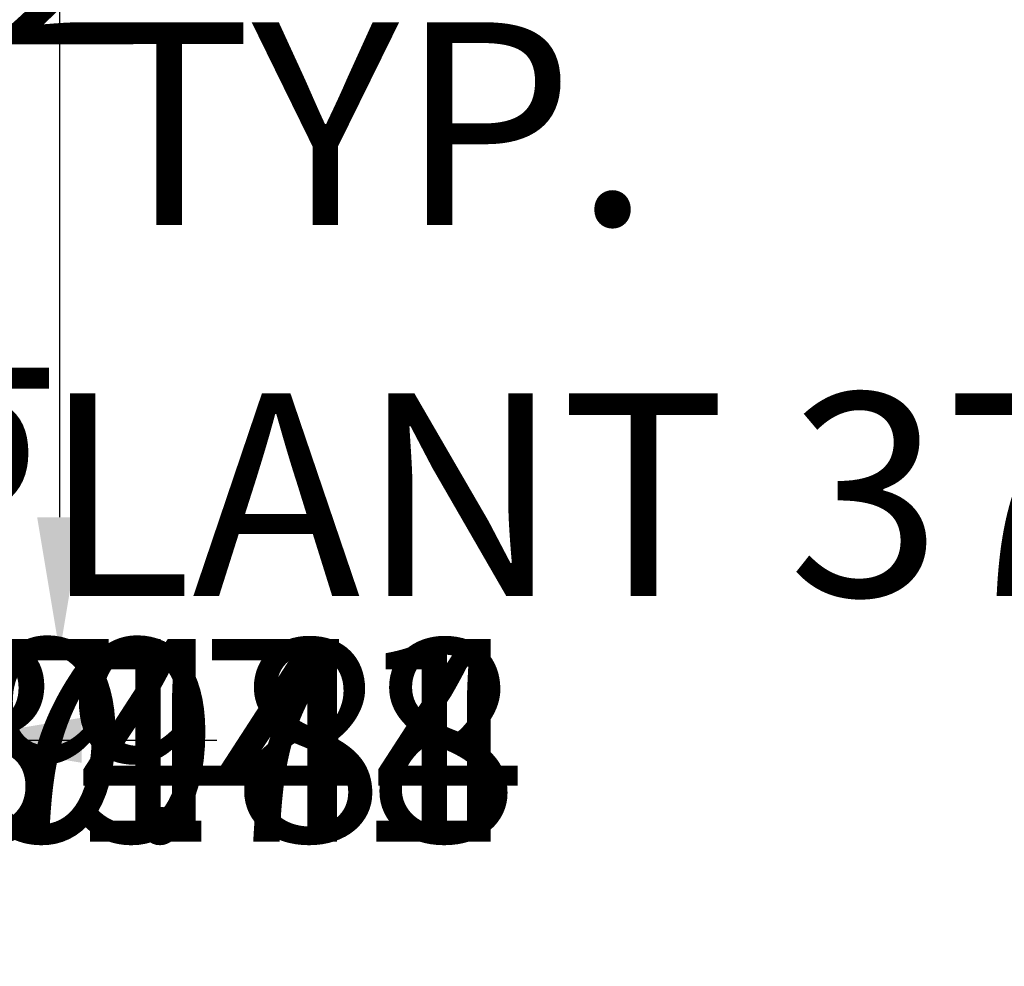
# Model space of a CAD drawing. Units: inches. Extents: x -307 to 2141, y -58 to 895.
# Tile 26 of 28: x 933 to 1283, y -44 to 292. Entities that reach past the tile are written whole.
import ezdxf

# ---------------------------------------------------------------- set-up
doc = ezdxf.new("R2010")
doc.units = ezdxf.units.IN
doc.header["$MEASUREMENT"] = 0
doc.layers.add('A-ANNO-DIMS', color=2, linetype='Continuous', lineweight=18)
doc.styles.get("Standard").update_dxf_attribs({"font": 'arial.ttf'})
doc.dimstyles.get("Standard").update_dxf_attribs({"dimtxt": 72, "dimasz": 48, "dimexe": 0.18, "dimexo": 0.0625, "dimgap": 0.09, "dimtad": 0, "dimtih": 1, "dimtoh": 1, "dimdec": 0, "dimrnd": 48, "dimzin": 0, "dimdsep": 46, "dimlunit": 3, "dimtxsty": 'Standard', "dimcen": 0.09, "dimadec": 0, "dimazin": 0, "dimtfac": 1, "dimtdec": 0, "dimtofl": 0, "dimtmove": 0, "dimatfit": 3, "dimfxl": 1, "dimtolj": 1, "dimtzin": 0, "dimarcsym": 0})

# ---------------------------------------------------------------- blocks, each defined once
blk = doc.blocks.new('*D34')
at = {"layer": 'A-ANNO-DIMS', "color": 0, "lineweight": -2, "transparency": 16777216}
for p, q in [((927.14, 490.97), (927.14, 538.97)), ((927.14, 538.97), (975.14, 538.97)), ((916.4, 442.97), (927.32, 442.97)), ((916.4, 370.95), (927.32, 370.95)), ((927.14, 322.95), (927.14, 274.95))]:
    blk.add_line(p, q, dxfattribs=at)
at = {"layer": 'A-ANNO-DIMS', "color": 0, "transparency": 16777216}
for points in [[(919.14, 490.97), (935.14, 490.97), (927.14, 442.97)], [(919.14, 322.95), (935.14, 322.95), (927.14, 370.95)]]:
    blk.add_solid(points, dxfattribs=at)
at = {"layer": 'Defpoints', "color": 0, "transparency": 16777216}
for p in [(916.34, 442.97), (927.14, 442.97), (916.34, 370.95)]:
    blk.add_point(p, dxfattribs=at)
at = {"layer": 'A-ANNO-DIMS', "color": 0, "transparency": 16777216, "insert": (1584.53, 538.97), "char_height": 72, "attachment_point": 5}
blk.add_mtext('\\A1;PAIRED WINDOW 72 TYP.', dxfattribs=at)
blk = doc.blocks.new('*D40')
at = {"layer": 'A-ANNO-DIMS', "color": 0, "lineweight": -2, "transparency": 16777216}
for p, q in [((725.38, 128.89), (725.38, 123.17)), ((762.77, 128.89), (762.77, 123.17)), ((677.38, 123.35), (629.38, 123.35)), ((810.77, 123.35), (858.77, 123.35))]:
    blk.add_line(p, q, dxfattribs=at)
at = {"layer": 'A-ANNO-DIMS', "color": 0, "transparency": 16777216}
for points in [[(677.38, 131.35), (677.38, 115.35), (725.38, 123.35)], [(810.77, 131.35), (810.77, 115.35), (762.77, 123.35)]]:
    blk.add_solid(points, dxfattribs=at)
at = {"layer": 'Defpoints', "color": 0, "transparency": 16777216}
for p in [(725.38, 128.96), (762.77, 128.96), (762.77, 123.35)]:
    blk.add_point(p, dxfattribs=at)
at = {"layer": 'A-ANNO-DIMS', "color": 0, "transparency": 16777216, "insert": (1208.37, 123.35), "char_height": 72, "attachment_point": 5}
blk.add_mtext('\\A1;PLANT 37 TYP.', dxfattribs=at)
blk = doc.blocks.new('*D41')
at = {"layer": 'A-ANNO-DIMS', "color": 0, "lineweight": -2, "transparency": 16777216}
for p, q in [((768.38, 207.13), (768.38, 255.13)), ((768.38, 255.13), (816.38, 255.13)), ((762.83, 159.13), (768.56, 159.13)), ((762.83, 128.96), (768.56, 128.96)), ((768.38, 80.96), (768.38, 32.96))]:
    blk.add_line(p, q, dxfattribs=at)
at = {"layer": 'A-ANNO-DIMS', "color": 0, "transparency": 16777216}
for points in [[(760.38, 207.13), (776.38, 207.13), (768.38, 159.13)], [(760.38, 80.96), (776.38, 80.96), (768.38, 128.96)]]:
    blk.add_solid(points, dxfattribs=at)
at = {"layer": 'Defpoints', "color": 0, "transparency": 16777216}
for p in [(762.77, 159.13), (768.38, 159.13), (762.77, 128.96)]:
    blk.add_point(p, dxfattribs=at)
at = {"layer": 'A-ANNO-DIMS', "color": 0, "transparency": 16777216, "insert": (991.68, 255.13), "char_height": 72, "attachment_point": 5}
blk.add_mtext('\\A1;30 TYP.', dxfattribs=at)
blk = doc.blocks.new('*D49')
at = {"layer": 'A-ANNO-DIMS', "color": 0, "lineweight": -2, "transparency": 16777216}
for p, q in [((733, 205.92), (733, 196.8)), ((754.34, 205.92), (754.34, 196.8)), ((685, 196.98), (637, 196.98)), ((802.34, 196.98), (850.34, 196.98))]:
    blk.add_line(p, q, dxfattribs=at)
at = {"layer": 'A-ANNO-DIMS', "color": 0, "transparency": 16777216}
for points in [[(685, 204.98), (685, 188.98), (733, 196.98)], [(802.34, 204.98), (802.34, 188.98), (754.34, 196.98)]]:
    blk.add_solid(points, dxfattribs=at)
at = {"layer": 'Defpoints', "color": 0, "transparency": 16777216}
for p in [(733, 205.98), (754.34, 205.98), (754.34, 196.98)]:
    blk.add_point(p, dxfattribs=at)
at = {"layer": 'A-ANNO-DIMS', "color": 0, "transparency": 16777216, "insert": (895.66, 196.98), "char_height": 72, "attachment_point": 5}
blk.add_mtext('\\A1;21', dxfattribs=at)
blk = doc.blocks.new('*D54')
at = {"layer": 'A-ANNO-DIMS', "color": 0, "lineweight": -2, "transparency": 16777216}
for p, q in [((605.34, 412.35), (605.34, 460.35)), ((605.34, 460.35), (653.34, 460.35)), ((596.4, 364.35), (605.52, 364.35)), ((596.4, 304.35), (605.52, 304.35)), ((605.34, 256.35), (605.34, 208.35))]:
    blk.add_line(p, q, dxfattribs=at)
at = {"layer": 'A-ANNO-DIMS', "color": 0, "transparency": 16777216}
for points in [[(597.34, 412.35), (613.34, 412.35), (605.34, 364.35)], [(597.34, 256.35), (613.34, 256.35), (605.34, 304.35)]]:
    blk.add_solid(points, dxfattribs=at)
at = {"layer": 'Defpoints', "color": 0, "transparency": 16777216}
for p in [(596.34, 364.35), (605.34, 364.35), (596.34, 304.35)]:
    blk.add_point(p, dxfattribs=at)
at = {"layer": 'A-ANNO-DIMS', "color": 0, "transparency": 16777216, "insert": (854, 460.35), "char_height": 72, "attachment_point": 5}
blk.add_mtext('\\A1;DESK 60', dxfattribs=at)
blk = doc.blocks.new('*D60')
at = {"layer": 'A-ANNO-DIMS', "color": 0, "lineweight": -2, "transparency": 16777216}
for p, q in [((659.86, 294.95), (659.86, 342.95)), ((659.86, 342.95), (707.86, 342.95)), ((663.34, 246.95), (659.68, 246.95)), ((663.34, 223.32), (659.68, 223.32)), ((659.86, 175.32), (659.86, 127.32))]:
    blk.add_line(p, q, dxfattribs=at)
at = {"layer": 'A-ANNO-DIMS', "color": 0, "transparency": 16777216}
for points in [[(651.86, 294.95), (667.86, 294.95), (659.86, 246.95)], [(651.86, 175.32), (667.86, 175.32), (659.86, 223.32)]]:
    blk.add_solid(points, dxfattribs=at)
at = {"layer": 'Defpoints', "color": 0, "transparency": 16777216}
for p in [(659.86, 246.95), (663.4, 246.95), (663.4, 223.32)]:
    blk.add_point(p, dxfattribs=at)
at = {"layer": 'A-ANNO-DIMS', "color": 0, "transparency": 16777216, "insert": (933.57, 342.95), "char_height": 72, "attachment_point": 5}
blk.add_mtext('\\A1;TABLE 24', dxfattribs=at)
blk = doc.blocks.new('*D63')
at = {"layer": 'A-ANNO-DIMS', "color": 0, "lineweight": -2, "transparency": 16777216}
for p, q in [((916.4, 691.34), (947.72, 691.34)), ((947.54, 643.34), (947.54, 416.19)), ((947.54, 115.34), (947.54, 342.49)), ((704.68, 67.34), (947.72, 67.34))]:
    blk.add_line(p, q, dxfattribs=at)
at = {"layer": 'A-ANNO-DIMS', "color": 0, "transparency": 16777216}
for points in [[(939.54, 643.34), (955.54, 643.34), (947.54, 691.34)], [(939.54, 115.34), (955.54, 115.34), (947.54, 67.34)]]:
    blk.add_solid(points, dxfattribs=at)
at = {"layer": 'Defpoints', "color": 0, "transparency": 16777216}
for p in [(916.34, 691.34), (704.62, 67.34), (947.54, 67.34)]:
    blk.add_point(p, dxfattribs=at)
at = {"layer": 'A-ANNO-DIMS', "color": 0, "transparency": 16777216, "insert": (947.54, 379.34), "char_height": 72, "attachment_point": 5}
blk.add_mtext('\\A1;624', dxfattribs=at)
blk = doc.blocks.new('*D72')
at = {"layer": 'A-ANNO-DIMS', "color": 0, "lineweight": -2, "transparency": 16777216}
for p, q in [((556.34, 91.28), (556.34, 35.96)), ((632.62, 91.28), (632.62, 35.96)), ((508.34, 36.14), (460.34, 36.14)), ((680.62, 36.14), (728.62, 36.14))]:
    blk.add_line(p, q, dxfattribs=at)
at = {"layer": 'A-ANNO-DIMS', "color": 0, "transparency": 16777216}
for points in [[(508.34, 44.14), (508.34, 28.14), (556.34, 36.14)], [(680.62, 44.14), (680.62, 28.14), (632.62, 36.14)]]:
    blk.add_solid(points, dxfattribs=at)
at = {"layer": 'Defpoints', "color": 0, "transparency": 16777216}
for p in [(556.34, 91.34), (632.62, 91.34), (632.62, 36.14)]:
    blk.add_point(p, dxfattribs=at)
at = {"layer": 'A-ANNO-DIMS', "color": 0, "transparency": 16777216, "insert": (849.97, 36.14), "char_height": 72, "attachment_point": 5}
blk.add_mtext('\\A1;76.29', dxfattribs=at)
blk = doc.blocks.new('*D74')
at = {"layer": 'A-ANNO-DIMS', "color": 0, "lineweight": -2, "transparency": 16777216}
for p, q in [((704.62, 91.28), (704.62, 35.96)), ((772.34, 91.28), (772.34, 35.96)), ((656.62, 36.14), (608.62, 36.14)), ((820.34, 36.14), (868.34, 36.14))]:
    blk.add_line(p, q, dxfattribs=at)
at = {"layer": 'A-ANNO-DIMS', "color": 0, "transparency": 16777216}
for points in [[(656.62, 44.14), (656.62, 28.14), (704.62, 36.14)], [(820.34, 44.14), (820.34, 28.14), (772.34, 36.14)]]:
    blk.add_solid(points, dxfattribs=at)
at = {"layer": 'Defpoints', "color": 0, "transparency": 16777216}
for p in [(704.62, 91.34), (772.34, 91.34), (772.34, 36.14)]:
    blk.add_point(p, dxfattribs=at)
at = {"layer": 'A-ANNO-DIMS', "color": 0, "transparency": 16777216, "insert": (983.15, 36.14), "char_height": 72, "attachment_point": 5}
blk.add_mtext('\\A1;67.71', dxfattribs=at)
blk = doc.blocks.new('*D84')
at = {"layer": 'A-ANNO-DIMS', "color": 0, "lineweight": -2, "transparency": 16777216}
for p, q in [((763.34, 472.28), (763.34, 35.96)), ((907.34, 472.28), (907.34, 35.96)), ((811.34, 36.14), (859.34, 36.14)), ((907.34, 36.14), (955.34, 36.14))]:
    blk.add_line(p, q, dxfattribs=at)
at = {"layer": 'A-ANNO-DIMS', "color": 0, "transparency": 16777216}
for points in [[(811.34, 44.14), (811.34, 28.14), (763.34, 36.14)], [(859.34, 44.14), (859.34, 28.14), (907.34, 36.14)]]:
    blk.add_solid(points, dxfattribs=at)
at = {"layer": 'Defpoints', "color": 0, "transparency": 16777216}
for p in [(763.34, 472.34), (907.34, 472.34), (907.34, 36.14)]:
    blk.add_point(p, dxfattribs=at)
at = {"layer": 'A-ANNO-DIMS', "color": 0, "transparency": 16777216, "insert": (1031.43, 36.14), "char_height": 72, "attachment_point": 5}
blk.add_mtext('\\A1;144', dxfattribs=at)
blk = doc.blocks.new('*D93')
at = {"layer": 'A-ANNO-DIMS', "color": 0, "lineweight": -2, "transparency": 16777216}
for p, q in [((859.34, 175.28), (859.34, 35.96)), ((907.34, 175.28), (907.34, 35.96)), ((811.34, 36.14), (763.34, 36.14)), ((955.34, 36.14), (1003.34, 36.14))]:
    blk.add_line(p, q, dxfattribs=at)
at = {"layer": 'A-ANNO-DIMS', "color": 0, "transparency": 16777216}
for points in [[(811.34, 44.14), (811.34, 28.14), (859.34, 36.14)], [(955.34, 44.14), (955.34, 28.14), (907.34, 36.14)]]:
    blk.add_solid(points, dxfattribs=at)
at = {"layer": 'Defpoints', "color": 0, "transparency": 16777216}
for p in [(859.34, 175.34), (907.34, 175.34), (907.34, 36.14)]:
    blk.add_point(p, dxfattribs=at)
at = {"layer": 'A-ANNO-DIMS', "color": 0, "transparency": 16777216, "insert": (1056.52, 36.14), "char_height": 72, "attachment_point": 5}
blk.add_mtext('\\A1;48', dxfattribs=at)
blk = doc.blocks.new('*D99')
at = {"layer": 'A-ANNO-DIMS', "color": 0, "lineweight": -2, "transparency": 16777216}
for p, q in [((763.34, 481.28), (763.34, 35.96)), ((802.34, 481.28), (802.34, 35.96)), ((715.34, 36.14), (667.34, 36.14)), ((850.34, 36.14), (898.34, 36.14))]:
    blk.add_line(p, q, dxfattribs=at)
at = {"layer": 'A-ANNO-DIMS', "color": 0, "transparency": 16777216}
for points in [[(715.34, 44.14), (715.34, 28.14), (763.34, 36.14)], [(850.34, 44.14), (850.34, 28.14), (802.34, 36.14)]]:
    blk.add_solid(points, dxfattribs=at)
at = {"layer": 'Defpoints', "color": 0, "transparency": 16777216}
for p in [(763.34, 481.34), (802.34, 481.34), (802.34, 36.14)]:
    blk.add_point(p, dxfattribs=at)
at = {"layer": 'A-ANNO-DIMS', "color": 0, "transparency": 16777216, "insert": (950.04, 36.14), "char_height": 72, "attachment_point": 5}
blk.add_mtext('\\A1;39', dxfattribs=at)
blk = doc.blocks.new('*D104')
at = {"layer": 'A-ANNO-DIMS', "color": 0, "lineweight": -2, "transparency": 16777216}
for p, q in [((885.13, 418.95), (885.13, 466.95)), ((885.13, 466.95), (933.13, 466.95)), ((916.27, 370.95), (884.95, 370.95)), ((916.27, 307.34), (884.95, 307.34)), ((885.13, 259.34), (885.13, 211.34))]:
    blk.add_line(p, q, dxfattribs=at)
at = {"layer": 'A-ANNO-DIMS', "color": 0, "transparency": 16777216}
for points in [[(877.13, 418.95), (893.13, 418.95), (885.13, 370.95)], [(877.13, 259.34), (893.13, 259.34), (885.13, 307.34)]]:
    blk.add_solid(points, dxfattribs=at)
at = {"layer": 'Defpoints', "color": 0, "transparency": 16777216}
for p in [(885.13, 370.95), (916.34, 370.95), (916.34, 307.34)]:
    blk.add_point(p, dxfattribs=at)
at = {"layer": 'A-ANNO-DIMS', "color": 0, "transparency": 16777216, "insert": (1047.95, 466.95), "char_height": 72, "attachment_point": 5}
blk.add_mtext('\\A1;63.61', dxfattribs=at)
blk = doc.blocks.new('*D105')
at = {"layer": 'A-ANNO-DIMS', "color": 0, "lineweight": -2, "transparency": 16777216}
for p, q in [((828.13, 271.34), (828.13, 319.34)), ((828.13, 319.34), (876.13, 319.34)), ((859.27, 223.34), (827.95, 223.34)), ((859.27, 211.34), (827.95, 211.34)), ((828.13, 163.34), (828.13, 115.34))]:
    blk.add_line(p, q, dxfattribs=at)
at = {"layer": 'A-ANNO-DIMS', "color": 0, "transparency": 16777216}
for points in [[(820.13, 271.34), (836.13, 271.34), (828.13, 223.34)], [(820.13, 163.34), (836.13, 163.34), (828.13, 211.34)]]:
    blk.add_solid(points, dxfattribs=at)
at = {"layer": 'Defpoints', "color": 0, "transparency": 16777216}
for p in [(828.13, 223.34), (859.34, 223.34), (859.34, 211.34)]:
    blk.add_point(p, dxfattribs=at)
at = {"layer": 'A-ANNO-DIMS', "color": 0, "transparency": 16777216, "insert": (924.03, 319.34), "char_height": 72, "attachment_point": 5}
blk.add_mtext('\\A1;12', dxfattribs=at)
blk = doc.blocks.new('*D106')
at = {"layer": 'A-ANNO-DIMS', "color": 0, "lineweight": -2, "transparency": 16777216}
for p, q in [((811.34, 166.28), (811.34, 35.96)), ((859.34, 166.28), (859.34, 35.96)), ((763.34, 36.14), (715.34, 36.14)), ((907.34, 36.14), (955.34, 36.14))]:
    blk.add_line(p, q, dxfattribs=at)
at = {"layer": 'A-ANNO-DIMS', "color": 0, "transparency": 16777216}
for points in [[(763.34, 44.14), (763.34, 28.14), (811.34, 36.14)], [(907.34, 44.14), (907.34, 28.14), (859.34, 36.14)]]:
    blk.add_solid(points, dxfattribs=at)
at = {"layer": 'Defpoints', "color": 0, "transparency": 16777216}
for p in [(811.34, 166.34), (859.34, 166.34), (859.34, 36.14)]:
    blk.add_point(p, dxfattribs=at)
at = {"layer": 'A-ANNO-DIMS', "color": 0, "transparency": 16777216, "insert": (1008.52, 36.14), "char_height": 72, "attachment_point": 5}
blk.add_mtext('\\A1;48', dxfattribs=at)

msp = doc.modelspace()

# ---------------------------------------------------------------- dimensions: what is measured, and where the dimension line sits
at = {"layer": 'A-ANNO-DIMS'}
for base, p1, p2, text, picture, middle in [((927.1381, 442.9669), (916.3358, 370.9517), (916.3358, 442.9669), 'PAIRED WINDOW <> TYP.', '*D34', (1584.5269, 538.9669)), ((605.3358, 364.3488), (596.3358, 304.3488), (596.3358, 364.3488), 'DESK <>', '*D54', (854.0043, 460.3488)), ((659.8571, 246.9465), (663.4018, 223.3153), (663.4018, 246.9465), 'TABLE <>', '*D60', (933.5733, 342.9465)), ((768.3792, 159.1282), (762.7703, 128.9569), (762.7703, 159.1282), '<> TYP.', '*D41', (991.6806, 255.1282))]:
    dim = msp.add_linear_dim(base=base, p1=p1, p2=p2, angle=90, text=text, dimstyle='Standard', override={"dimdec": 0, "dimlfac": 1, "dimrnd": 0, "dimzin": 0, "dimdsep": 46, "dimlunit": 2}, dxfattribs=at)
    dim.commit()
    dim.dimension.update_dxf_attribs({"geometry": picture, "text_midpoint": middle})
for base, p1, p2, override, picture, middle in [((947.5398, 67.3408), (916.3358, 691.3408), (704.6211, 67.3408), {"dimdec": 0, "dimlfac": 1, "dimrnd": 0, "dimzin": 0, "dimdsep": 46, "dimlunit": 2}, '*D63', (947.5398, 379.3408)), ((885.1318, 370.9517), (916.3358, 307.3408), (916.3358, 370.9517), {"dimdec": 2, "dimlfac": 1, "dimrnd": 0, "dimzin": 0, "dimdsep": 46, "dimlunit": 2}, '*D104', (1047.9504, 466.9517)), ((828.1318, 223.3408), (859.3358, 211.3408), (859.3358, 223.3408), {"dimdec": 0, "dimlfac": 1, "dimrnd": 0, "dimzin": 0, "dimdsep": 46, "dimlunit": 2}, '*D105', (924.0336, 319.3408))]:
    dim = msp.add_linear_dim(base=base, p1=p1, p2=p2, angle=90, dimstyle='Standard', override=override, dxfattribs=at)
    dim.commit()
    dim.dimension.update_dxf_attribs({"geometry": picture, "text_midpoint": middle})
for base, p1, p2, override, picture, middle in [((802.3358, 36.1368), (763.3358, 481.3408), (802.3358, 481.3408), {"dimdec": 0, "dimlfac": 1, "dimrnd": 0, "dimzin": 0, "dimdsep": 46, "dimlunit": 2}, '*D99', (950.0438, 36.1368)), ((907.3358, 36.1368), (763.3358, 472.3408), (907.3358, 472.3408), {"dimdec": 0, "dimlfac": 1, "dimrnd": 0, "dimzin": 0, "dimdsep": 46, "dimlunit": 2}, '*D84', (1031.4286, 36.1368)), ((754.3358, 196.9815), (733.0025, 205.9815), (754.3358, 205.9815), {"dimdec": 0, "dimlfac": 1, "dimrnd": 0, "dimzin": 0, "dimdsep": 46, "dimlunit": 2}, '*D49', (895.6591, 196.9815)), ((907.3358, 36.1368), (859.3358, 175.3408), (907.3358, 175.3408), {"dimdec": 0, "dimlfac": 1, "dimrnd": 0, "dimzin": 0, "dimdsep": 46, "dimlunit": 2}, '*D93', (1056.5172, 36.1368)), ((859.3358, 36.1368), (811.3358, 166.3408), (859.3358, 166.3408), {"dimdec": 0, "dimlfac": 1, "dimrnd": 0, "dimzin": 0, "dimdsep": 46, "dimlunit": 2}, '*D106', (1008.5172, 36.1368)), ((632.6211, 36.1368), (556.3358, 91.3408), (632.6211, 91.3408), {"dimdec": 2, "dimlfac": 1, "dimrnd": 0, "dimzin": 0, "dimdsep": 46, "dimlunit": 2}, '*D72', (849.9716, 36.1368)), ((772.3358, 36.1368), (704.6211, 91.3408), (772.3358, 91.3408), {"dimdec": 2, "dimlfac": 1, "dimrnd": 0, "dimzin": 0, "dimdsep": 46, "dimlunit": 2}, '*D74', (983.1544, 36.1368))]:
    dim = msp.add_linear_dim(base=base, p1=p1, p2=p2, dimstyle='Standard', override=override, dxfattribs=at)
    dim.commit()
    dim.dimension.update_dxf_attribs({"geometry": picture, "text_midpoint": middle})
dim = msp.add_linear_dim(base=(762.7703, 123.348), p1=(725.3775, 128.9569), p2=(762.7703, 128.9569), text='PLANT <> TYP.', dimstyle='Standard', override={"dimdec": 0, "dimlfac": 1, "dimrnd": 0, "dimzin": 0, "dimdsep": 46, "dimlunit": 2}, dxfattribs=at)
dim.commit()
dim.dimension.update_dxf_attribs({"geometry": '*D40', "text_midpoint": (1208.3746, 123.348)})

doc.saveas('drawing.dxf')
